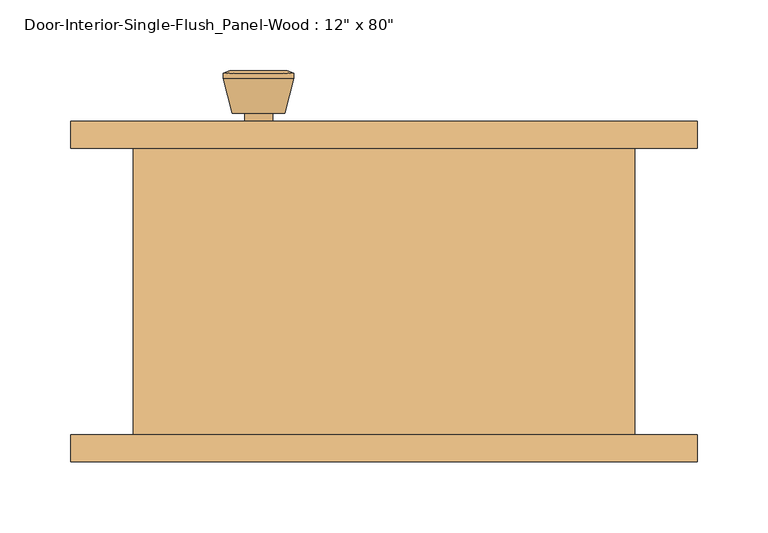
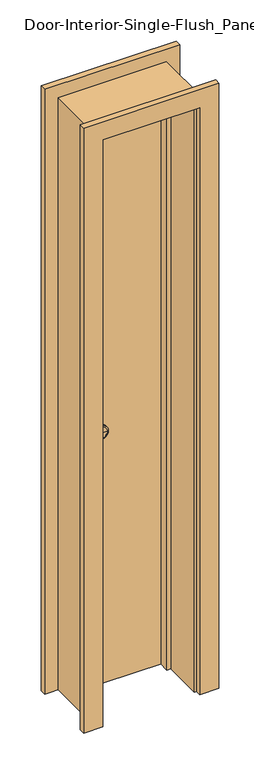
"""IFC4 building model written with IfcOpenShell, lengths in millimetres: door geometry."""

from ifc_helpers import new_model, si_unit, point, frame, frame_2d, origin, origin_with_axes, place, context, project, spatial, polyline, circle_curve, trimmed, segment, composite_curve, outline, extrude, faceted_brep, source, transform, mapped, element, save
from ifc_brep_helpers import plane_surface, cylinder_surface, revolved_surface, advanced_brep


def door_b2d2822a(model_context):
    return source(origin(), model_context, "Body", "SolidModel", [
        advanced_brep(
        [(-88.9, 57.5, 914.4), (-78.9, 57.5, 914.4), (-98.9, 57.5, 914.4), (-68.4241324, 8.5, 914.4), (-88.9, 8.5, 914.4), (-109.3758676, 8.5, 914.4), (-63.9, 10.3278681, 914.4), (-113.9, 10.3278681, 914.4), (-63.9, 13.7915463, 914.4), (-113.9, 13.7915463, 914.4), (-70.263764, 38.5, 914.4), (-107.536236, 38.5, 914.4), (-78.9, 38.5, 914.4), (-98.9, 38.5, 914.4)],
        [
            (0, 1),
            (1, 2, circle_curve(frame((-88.9, 57.5, 914.4), z_axis=(0.0, 1.0, 0.0), x_axis=(-1.0, 0.0, 0.0)), 10.0)),
            (2, 0),
            (2, 1, circle_curve(frame((-88.9, 57.5, 914.4), z_axis=(0.0, 1.0, 0.0), x_axis=(-1.0, 0.0, 0.0)), 10.0)),
            (3, 4),
            (4, 5),
            (5, 3, circle_curve(frame((-88.9, 8.5, 914.4), z_axis=(0.0, -1.0, 0.0), x_axis=(-1.0, 0.0, 0.0)), 20.4758676)),
            (3, 5, circle_curve(frame((-88.9, 8.5, 914.4), z_axis=(0.0, -1.0, 0.0), x_axis=(-1.0, 0.0, 0.0)), 20.4758676)),
            (6, 3),
            (5, 7),
            (7, 6, circle_curve(frame((-88.9, 10.3278681, 914.4), z_axis=(0.0, -1.0, 0.0), x_axis=(-1.0, 0.0, 0.0)), 25.0)),
            (6, 7, circle_curve(frame((-88.9, 10.3278681, 914.4), z_axis=(0.0, -1.0, 0.0), x_axis=(-1.0, 0.0, 0.0)), 25.0)),
            (8, 6),
            (7, 9),
            (9, 8, circle_curve(frame((-88.9, 13.7915463, 914.4), z_axis=(0.0, -1.0, 0.0), x_axis=(-1.0, 0.0, 0.0)), 25.0)),
            (8, 9, circle_curve(frame((-88.9, 13.7915463, 914.4), z_axis=(0.0, -1.0, 0.0), x_axis=(-1.0, 0.0, 0.0)), 25.0)),
            (10, 8),
            (9, 11),
            (11, 10, circle_curve(frame((-88.9, 38.5, 914.4), z_axis=(0.0, -1.0, 0.0), x_axis=(-1.0, 0.0, 0.0)), 18.636236)),
            (10, 11, circle_curve(frame((-88.9, 38.5, 914.4), z_axis=(0.0, -1.0, 0.0), x_axis=(-1.0, 0.0, 0.0)), 18.636236)),
            (12, 10),
            (11, 13),
            (13, 12, circle_curve(frame((-88.9, 38.5, 914.4), z_axis=(0.0, -1.0, 0.0), x_axis=(-1.0, 0.0, 0.0)), 10.0)),
            (12, 13, circle_curve(frame((-88.9, 38.5, 914.4), z_axis=(0.0, -1.0, 0.0), x_axis=(-1.0, 0.0, 0.0)), 10.0)),
            (1, 12),
            (13, 2),
        ],
        [
            plane_surface(frame((-88.9, 57.5, 914.4), z_axis=(0.0, 1.0, 0.0), x_axis=(-1.0, 0.0, 0.0))),
            plane_surface(frame((-88.9, 8.5, 914.4), z_axis=(0.0, -1.0, 0.0), x_axis=(-1.0, 0.0, 0.0))),
            revolved_surface(polyline([(-109.3758676, 8.5, 914.4), (-113.9, 10.3278681, 914.4)]), (-88.9, 57.5, 914.4), (0.0, 1.0, 0.0)),
            cylinder_surface(frame((-88.9, 57.5, 914.4), z_axis=(0.0, 1.0, 0.0), x_axis=(-1.0, 0.0, 0.0)), 25.0),
            revolved_surface(polyline([(-113.9, 13.7915463, 914.4), (-107.536236, 38.5, 914.4)]), (-88.9, 57.5, 914.4), (0.0, 1.0, 0.0)),
            plane_surface(frame((-88.9, 38.5, 914.4), z_axis=(0.0, 1.0, 0.0), x_axis=(-1.0, 0.0, 0.0))),
            cylinder_surface(frame((-88.9, 57.5, 914.4), z_axis=(0.0, 1.0, 0.0), x_axis=(-1.0, 0.0, 0.0)), 10.0),
        ],
        [
            (0, [[1, 2, 3]]),
            (0, [[-3, 4, -1]]),
            (1, [[5, 6, 7]]),
            (1, [[-6, -5, 8]]),
            (2, [[9, -7, 10, 11]]),
            (2, [[-10, -8, -9, 12]]),
            (3, [[13, -11, 14, 15]]),
            (3, [[-14, -12, -13, 16]]),
            (4, [[17, -15, 18, 19]]),
            (4, [[-18, -16, -17, 20]]),
            (5, [[21, -19, 22, 23]]),
            (5, [[-22, -20, -21, 24]]),
            (6, [[25, -23, 26, -2]]),
            (6, [[-26, -24, -25, -4]]),
        ],
    ),
        extrude(outline(composite_curve([segment(trimmed(circle_curve(frame_2d((914.4, -88.9)), 30.0), [point((914.4, -118.9))], [point((914.4, -58.9))], False, "CARTESIAN"), True, "CONTINUOUS"), segment(trimmed(circle_curve(frame_2d((914.4, -88.9)), 30.0), [point((914.4, -58.9))], [point((914.4, -118.9))], False, "CARTESIAN"), True, "CONTINUOUS")], self_intersect=False)), frame((0.0, 57.5, 0.0), z_axis=(0.0, 1.0, 0.0), x_axis=(0.0, 0.0, 1.0)), (0.0, 0.0, 1.0), 6.0),
        advanced_brep(
        [(-88.9, 104.425, 914.4), (-98.9, 104.425, 914.4), (-78.9, 104.425, 914.4), (-68.4241324, 153.425, 914.4), (-109.3758676, 153.425, 914.4), (-88.9, 153.425, 914.4), (-63.9, 151.5971319, 914.4), (-113.9, 151.5971319, 914.4), (-63.9, 148.1334537, 914.4), (-113.9, 148.1334537, 914.4), (-70.263764, 123.425, 914.4), (-107.536236, 123.425, 914.4), (-78.9, 123.425, 914.4), (-98.9, 123.425, 914.4)],
        [
            (0, 1),
            (1, 2, circle_curve(frame((-88.9, 104.425, 914.4), z_axis=(0.0, -1.0, 0.0), x_axis=(-1.0, 0.0, 0.0)), 10.0)),
            (2, 0),
            (2, 1, circle_curve(frame((-88.9, 104.425, 914.4), z_axis=(0.0, -1.0, 0.0), x_axis=(-1.0, 0.0, 0.0)), 10.0)),
            (3, 4, circle_curve(frame((-88.9, 153.425, 914.4), z_axis=(0.0, 1.0, 0.0), x_axis=(-1.0, 0.0, 0.0)), 20.4758676)),
            (4, 5),
            (5, 3),
            (4, 3, circle_curve(frame((-88.9, 153.425, 914.4), z_axis=(0.0, 1.0, 0.0), x_axis=(-1.0, 0.0, 0.0)), 20.4758676)),
            (6, 7, circle_curve(frame((-88.9, 151.5971319, 914.4), z_axis=(0.0, 1.0, 0.0), x_axis=(-1.0, 0.0, 0.0)), 25.0)),
            (7, 4),
            (3, 6),
            (7, 6, circle_curve(frame((-88.9, 151.5971319, 914.4), z_axis=(0.0, 1.0, 0.0), x_axis=(-1.0, 0.0, 0.0)), 25.0)),
            (8, 9, circle_curve(frame((-88.9, 148.1334537, 914.4), z_axis=(0.0, 1.0, 0.0), x_axis=(-1.0, 0.0, 0.0)), 25.0)),
            (9, 7),
            (6, 8),
            (9, 8, circle_curve(frame((-88.9, 148.1334537, 914.4), z_axis=(0.0, 1.0, 0.0), x_axis=(-1.0, 0.0, 0.0)), 25.0)),
            (10, 11, circle_curve(frame((-88.9, 123.425, 914.4), z_axis=(0.0, 1.0, 0.0), x_axis=(-1.0, 0.0, 0.0)), 18.636236)),
            (11, 9),
            (8, 10),
            (11, 10, circle_curve(frame((-88.9, 123.425, 914.4), z_axis=(0.0, 1.0, 0.0), x_axis=(-1.0, 0.0, 0.0)), 18.636236)),
            (12, 13, circle_curve(frame((-88.9, 123.425, 914.4), z_axis=(0.0, 1.0, 0.0), x_axis=(-1.0, 0.0, 0.0)), 10.0)),
            (13, 11),
            (10, 12),
            (13, 12, circle_curve(frame((-88.9, 123.425, 914.4), z_axis=(0.0, 1.0, 0.0), x_axis=(-1.0, 0.0, 0.0)), 10.0)),
            (1, 13),
            (12, 2),
        ],
        [
            plane_surface(frame((-88.9, 104.425, 914.4), z_axis=(0.0, -1.0, 0.0), x_axis=(-1.0, 0.0, 0.0))),
            plane_surface(frame((-88.9, 153.425, 914.4), z_axis=(0.0, 1.0, 0.0), x_axis=(-1.0, 0.0, 0.0))),
            revolved_surface(polyline([(-109.3758676, 153.425, 914.4), (-113.9, 151.5971319, 914.4)]), (-88.9, 104.425, 914.4), (0.0, -1.0, 0.0)),
            cylinder_surface(frame((-88.9, 104.425, 914.4), z_axis=(0.0, -1.0, 0.0), x_axis=(-1.0, 0.0, 0.0)), 25.0),
            revolved_surface(polyline([(-113.9, 148.1334537, 914.4), (-107.536236, 123.425, 914.4)]), (-88.9, 104.425, 914.4), (0.0, -1.0, 0.0)),
            plane_surface(frame((-88.9, 123.425, 914.4), z_axis=(0.0, -1.0, 0.0), x_axis=(-1.0, 0.0, 0.0))),
            cylinder_surface(frame((-88.9, 104.425, 914.4), z_axis=(0.0, -1.0, 0.0), x_axis=(-1.0, 0.0, 0.0)), 10.0),
        ],
        [
            (0, [[1, 2, 3]]),
            (0, [[-3, 4, -1]]),
            (1, [[5, 6, 7]]),
            (1, [[8, -7, -6]]),
            (2, [[9, 10, -5, 11]]),
            (2, [[12, -11, -8, -10]]),
            (3, [[13, 14, -9, 15]]),
            (3, [[16, -15, -12, -14]]),
            (4, [[17, 18, -13, 19]]),
            (4, [[20, -19, -16, -18]]),
            (5, [[21, 22, -17, 23]]),
            (5, [[24, -23, -20, -22]]),
            (6, [[-2, 25, -21, 26]]),
            (6, [[-4, -26, -24, -25]]),
        ],
    ),
        extrude(outline(composite_curve([segment(trimmed(circle_curve(frame_2d((914.4, -88.9)), 30.0), [point((914.4, -118.9))], [point((914.4, -58.9))], False, "CARTESIAN"), True, "CONTINUOUS"), segment(trimmed(circle_curve(frame_2d((914.4, -88.9)), 30.0), [point((914.4, -58.9))], [point((914.4, -118.9))], False, "CARTESIAN"), True, "CONTINUOUS")], self_intersect=False)), frame((0.0, 98.425, 0.0), z_axis=(0.0, 1.0, 0.0), x_axis=(0.0, 0.0, 1.0)), (0.0, 0.0, 1.0), 6.0),
        extrude(outline(polyline([(152.4, 63.5), (-152.4, 63.5), (-152.4, 98.425), (152.4, 98.425), (152.4, 63.5)])), origin_with_axes(), (0.0, 0.0, 1.0), 2032.0),
        faceted_brep([(177.8, 98.425, 0.0), (177.8, -104.775, 0.0), (152.4, -104.775, 0.0), (152.4, 28.575, 0.0), (139.7, 28.575, 0.0), (139.7, 63.5, 0.0), (152.4, 63.5, 0.0), (152.4, 98.425, 0.0), (177.8, 98.425, 2057.4), (177.8, -104.775, 2057.4), (-177.8, -104.775, 2057.4), (-177.8, -104.775, 0.0), (-152.4, -104.775, 0.0), (-152.4, -104.775, 2032.0), (152.4, -104.775, 2032.0), (152.4, 28.575, 2032.0), (-152.4, 28.575, 2032.0), (-152.4, 28.575, 0.0), (-139.7, 28.575, 0.0), (-139.7, 28.575, 2019.3), (139.7, 28.575, 2019.3), (139.7, 63.5, 2019.3), (-139.7, 63.5, 2019.3), (-139.7, 63.5, 0.0), (-152.4, 63.5, 0.0), (-152.4, 63.5, 2032.0), (152.4, 63.5, 2032.0), (152.4, 98.425, 2032.0), (-152.4, 98.425, 2032.0), (-152.4, 98.425, 0.0), (-177.8, 98.425, 0.0), (-177.8, 98.425, 2057.4)], [[[0, 1, 2, 3, 4, 5, 6, 7]], [[1, 0, 8, 9]], [[2, 1, 9, 10, 11, 12, 13, 14]], [[3, 2, 14, 15]], [[4, 3, 15, 16, 17, 18, 19, 20]], [[5, 4, 20, 21]], [[6, 5, 21, 22, 23, 24, 25, 26]], [[7, 6, 26, 27]], [[0, 7, 27, 28, 29, 30, 31, 8]], [[9, 8, 31, 10]], [[15, 14, 13, 16]], [[21, 20, 19, 22]], [[27, 26, 25, 28]], [[30, 29, 24, 23, 18, 17, 12, 11]], [[10, 31, 30, 11]], [[16, 13, 12, 17]], [[22, 19, 18, 23]], [[28, 25, 24, 29]]]),
        extrude(outline(polyline([(0.0, 158.75), (0.0, 222.25), (2101.85, 222.25), (2101.85, -222.25), (0.0, -222.25), (0.0, -158.75), (2038.35, -158.75), (2038.35, 158.75), (0.0, 158.75)])), frame((0.0, -123.825, 0.0), z_axis=(0.0, 1.0, 0.0), x_axis=(0.0, 0.0, 1.0)), (0.0, 0.0, 1.0), 19.05),
        extrude(outline(polyline([(0.0, 158.75), (0.0, 222.25), (2101.85, 222.25), (2101.85, -222.25), (0.0, -222.25), (0.0, -158.75), (2038.35, -158.75), (2038.35, 158.75), (0.0, 158.75)])), frame((0.0, 98.425, 0.0), z_axis=(0.0, 1.0, 0.0), x_axis=(0.0, 0.0, 1.0)), (0.0, 0.0, 1.0), 19.05),
    ])


if __name__ == "__main__":
    model = new_model("IFC4")
    model_context = context("Model", 3, world=origin())
    ifc_project = project(units=[si_unit("LENGTHUNIT", "METRE", prefix="MILLI")], contexts=[model_context])
    site = spatial("IfcSite", under=ifc_project)
    building = spatial("IfcBuilding", under=site)
    placement = place(None, origin())
    door_shape = door_b2d2822a(model_context)
    element("IfcDoor", 1, ObjectType="Door-Interior-Single-Flush_Panel-Wood : 12\" x 80\"", at=placement, inside=building, context=model_context, shape_type="MappedRepresentation", body=[
        mapped(door_shape, transform((0.0, 0.0, 0.0), x_axis=(1.0, 0.0, 0.0), y_axis=(0.0, 1.0, 0.0), z_axis=(0.0, 0.0, 1.0))),
    ])
    save(model, "model.ifc")

# Revit data of these elements
# Type "Door-Interior-Single-Flush_Panel-Wood : 12\" x 80\""
#   Type Mark = "10"
#   Assembly Code = "C1020300"
#   Analytic Construction = "Wooden"
#   Thickness = 0' - 1 3/8"
#   Thermal Resistance (R) = 2.5876 (h·ft²·°F)/BTU
#   Swing Angle [instance default] = 90.00°
#   Rough Width = 1' - 2"
#   Rough Height = 6' - 9"
#   Height = 6' - 8"
#   Width = 1' - 0"
#   Heat Transfer Coefficient (U) = 0.3865 BTU/(h·ft²·°F)
#   Trim Material = Cherry
#   Panel Material = Cherry
#   Frame Material = Cherry
#   Door Handle Material = Aluminum
#   Visual Light Transmittance = 0
#   Solar Heat Gain Coefficient = 0
#   Wall Closure = (empty or 0)
#   Function = (empty or 0)
# Element 1 (IfcDoor, "Door-Interior-Single-Flush_Panel-Wood : 12\" x 80\"")
#   Materials on its faces: "Cherry", "Aluminum"
# Materials
#   "Cherry": class "Wood", colour RGB 226 177 128, transparency 0, Description = "Prunus Serotina", Cost = 0
#   "Aluminum": class "Metal", colour RGB 247 247 247, transparency 0, Description = "Aluminum 6061", Cost = 0
